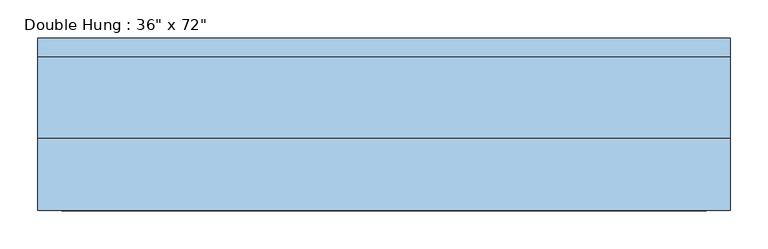
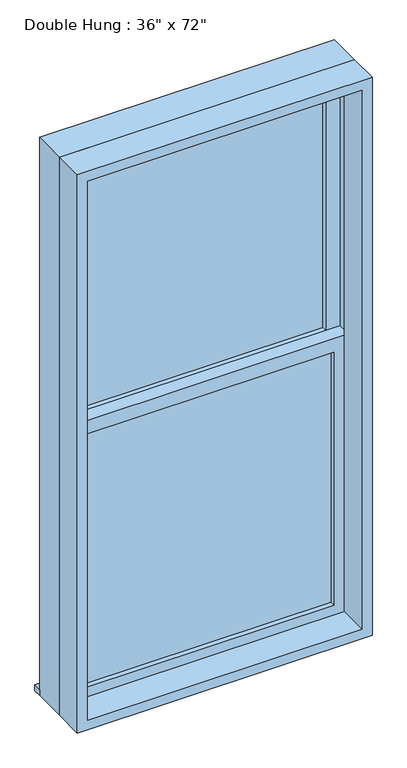
"""IFC4 building model written with IfcOpenShell, lengths in millimetres: window geometry."""

from ifc_helpers import new_model, si_unit, frame, origin, place, context, project, spatial, polyline, outline, extrude, source, transform, mapped, element, save


def window_f274a882(model_context):
    return source(origin(), model_context, "Body", "SweptSolid", [
        extrude(outline(polyline([(-393.7, 22.225), (393.7, 22.225), (393.7, 9.525), (-393.7, 9.525), (-393.7, 22.225)])), frame((0.0, 0.0, 368.3), z_axis=(0.0, 0.0, 1.0), x_axis=(1.0, 0.0, 0.0)), (0.0, 0.0, 1.0), 828.675),
        extrude(outline(polyline([(1241.425, -438.15), (323.85, -438.15), (323.85, 438.15), (1241.425, 438.15), (1241.425, -438.15)]), holes=[polyline([(1196.975, -393.7), (1196.975, 393.7), (368.3, 393.7), (368.3, -393.7), (1196.975, -393.7)])]), frame((0.0, -6.35, 0.0), z_axis=(0.0, 1.0, 0.0), x_axis=(0.0, 0.0, 1.0)), (0.0, 0.0, 1.0), 44.45),
        extrude(outline(polyline([(-457.2, 127.0), (457.2, 127.0), (457.2, 101.6), (-457.2, 101.6), (-457.2, 127.0)])), frame((0.0, 0.0, 304.8), z_axis=(0.0, 0.0, 1.0), x_axis=(1.0, 0.0, 0.0)), (0.0, 0.0, 1.0), 19.05),
        extrude(outline(polyline([(393.7, 53.975), (-393.7, 53.975), (-393.7, 66.675), (393.7, 66.675), (393.7, 53.975)])), frame((0.0, 0.0, 1241.425), z_axis=(0.0, 0.0, 1.0), x_axis=(1.0, 0.0, 0.0)), (0.0, 0.0, 1.0), 828.675),
        extrude(outline(polyline([(2114.55, -438.15), (1196.975, -438.15), (1196.975, 438.15), (2114.55, 438.15), (2114.55, -438.15)]), holes=[polyline([(2070.1, -393.7), (2070.1, 393.7), (1241.425, 393.7), (1241.425, -393.7), (2070.1, -393.7)])]), frame((0.0, 38.1, 0.0), z_axis=(0.0, 1.0, 0.0), x_axis=(0.0, 0.0, 1.0)), (0.0, 0.0, 1.0), 44.45),
        extrude(outline(polyline([(2133.6, -457.2), (304.8, -457.2), (304.8, 457.2), (2133.6, 457.2), (2133.6, -457.2)]), holes=[polyline([(2101.85, -425.45), (2101.85, 425.45), (336.55, 425.45), (336.55, -425.45), (2101.85, -425.45)])]), frame((0.0, -101.6, 0.0), z_axis=(0.0, 1.0, 0.0), x_axis=(0.0, 0.0, 1.0)), (0.0, 0.0, 1.0), 95.25),
        extrude(outline(polyline([(2133.6, 457.2), (2133.6, -457.2), (304.8, -457.2), (304.8, 457.2), (2133.6, 457.2)]), holes=[polyline([(2114.55, 438.15), (323.85, 438.15), (323.85, -438.15), (2114.55, -438.15), (2114.55, 438.15)])]), frame((0.0, -6.35, 0.0), z_axis=(0.0, 1.0, 0.0), x_axis=(0.0, 0.0, 1.0)), (0.0, 0.0, 1.0), 107.95),
    ])


if __name__ == "__main__":
    model = new_model("IFC4")
    model_context = context("Model", 3, world=origin())
    ifc_project = project(units=[si_unit("LENGTHUNIT", "METRE", prefix="MILLI")], contexts=[model_context])
    site = spatial("IfcSite", under=ifc_project)
    building = spatial("IfcBuilding", under=site)
    placement = place(None, origin())
    window_shape = window_f274a882(model_context)
    element("IfcWindow", 1, ObjectType="Double Hung : 36\" x 72\"", at=placement, inside=building, context=model_context, shape_type="MappedRepresentation", body=[
        mapped(window_shape, transform((0.0, 0.0, 0.0), x_axis=(1.0, 0.0, 0.0), y_axis=(0.0, 1.0, 0.0), z_axis=(0.0, 0.0, 1.0))),
    ])
    save(model, "model.ifc")

# Revit data of these elements
# Type "Double Hung : 36\" x 72\""
#   Type Mark = "18"
#   Construction Type Id = "GSP4R"
#   Assembly Code = "B2020100"
#   Analytic Construction = "1/8 in Pilkington single glazing"
#   Visual Light Transmittance = 0.9
#   Solar Heat Gain Coefficient = 0.78
#   Heat Transfer Coefficient (U) = 0.6496 BTU/(h·ft²·°F)
#   Height = 6' - 0"
#   Default Sill Height = 1' - 0"
#   Width = 3' - 0"
#   Window Inset = 0' - 0 3/4"
#   Define Thermal Properties by = 1
#   Glass Pane Material = Glass
#   Sash Material = Sash
#   Description = (empty or 0)
#   Wall Closure = (empty or 0)
# Element 1 (IfcWindow, "Double Hung : 36\" x 72\"")
#   Materials on its faces: "Sash", "Glass"
# Materials
#   "Glass": class "Glass", colour RGB 0 128 192, transparency 0.75, Description = "Soda Lime Glass", Cost = 0
#   "Sash": class "Wood", colour RGB 224 178 126, transparency 0
